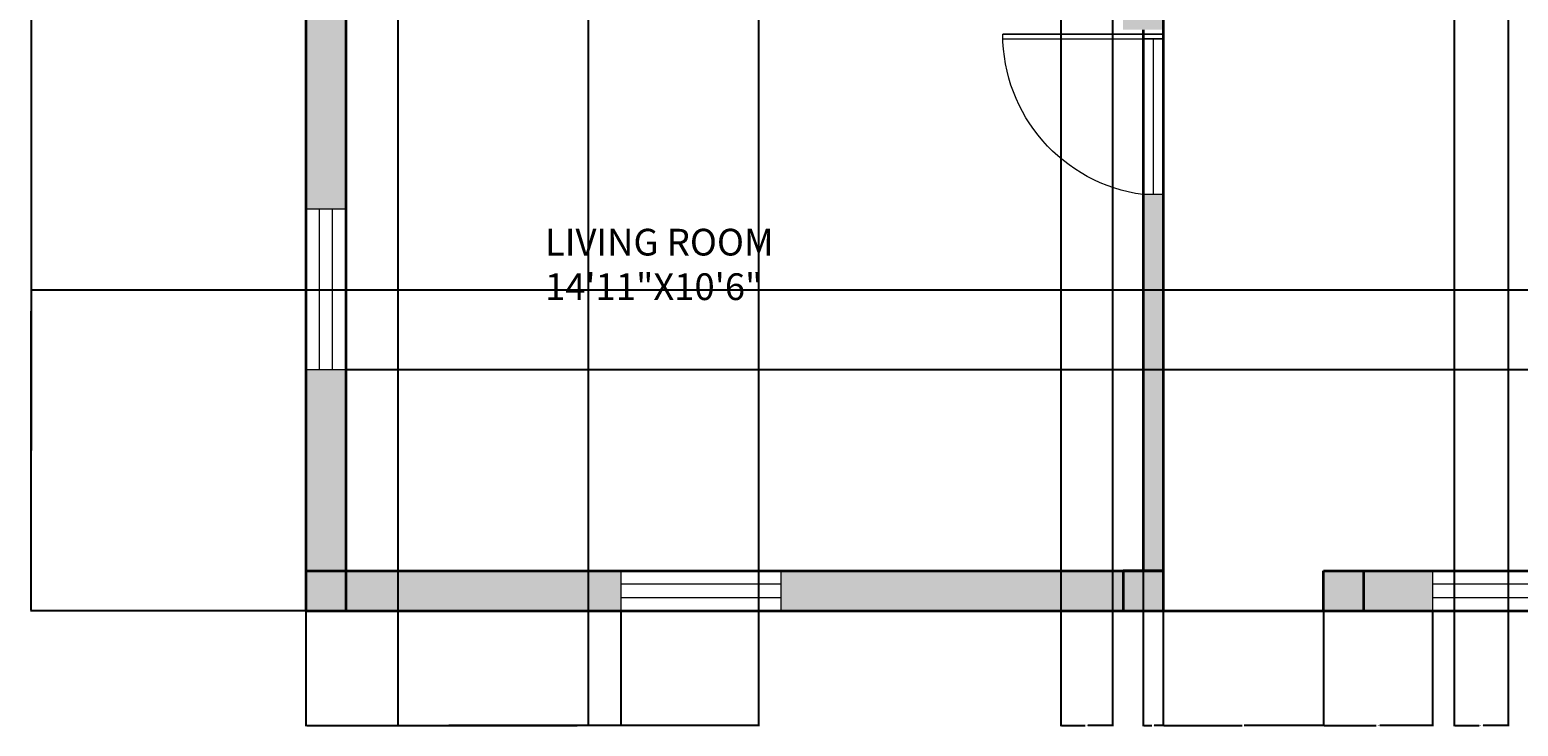
# Model space of a CAD drawing. Units: inches. Extents: x 6217 to 6782, y 16564 to 16973.
# Tile 1 of 3: x 6218 to 6552, y 16564 to 16720. Entities that reach past the tile are written whole.
import ezdxf

# ---------------------------------------------------------------- set-up
doc = ezdxf.new("R2010")
doc.units = ezdxf.units.IN
doc.header["$MEASUREMENT"] = 0
for name, color, linetype, lineweight in [('A-ANNO-DIMS', 2, 'Continuous', 18), ('A-AREA-IDEN', 7, 'Continuous', 18), ('A-COLS', 7, 'Continuous', 35), ('A-DOOR', 3, 'Continuous', 18), ('A-GLAZ', 4, 'Continuous', 18), ('A-WALL', 7, 'Continuous', 35)]:
    doc.layers.add(name, color=color, linetype=linetype, lineweight=lineweight)
doc.layers.add('A-COLS-PATT', color=252, linetype='Continuous', lineweight=13, true_color=0x939598)
doc.layers.add('A-WALL-PATT', color=146, linetype='Continuous', lineweight=13, true_color=0x105689)
doc.styles.get("Standard").update_dxf_attribs({"font": 'arial.ttf'})
doc.dimstyles.get("Standard").update_dxf_attribs({"dimtxt": 0.18, "dimasz": 0.18, "dimexe": 0.18, "dimexo": 0.0625, "dimgap": 0.09, "dimtad": 0, "dimtih": 1, "dimtoh": 1, "dimdec": 4, "dimzin": 0, "dimdsep": 46, "dimtxsty": 'Standard', "dimcen": 0.09, "dimadec": 0, "dimazin": 0, "dimtfac": 1, "dimtdec": 4, "dimtofl": 0, "dimtmove": 0, "dimatfit": 3, "dimfxl": 1, "dimtolj": 1, "dimtzin": 0, "dimarcsym": 0})

# ---------------------------------------------------------------- blocks, each defined once
blk = doc.blocks.new('WIN-36')
for p, q in [((0, 9), (0, 0)), ((36, 9), (0, 9)), ((36, 0), (36, 9)), ((36, 6), (0, 6)), ((0, 3), (36, 3)), ((0, 0), (36, 0))]:
    blk.add_line(p, q)
blk = doc.blocks.new('DOOR-SINGLE-36-A')
for p, q in [((0, 36), (-4.5, 36)), ((-2.25, 1), (-2.25, 36)), ((0, 0), (0, 36)), ((-36, 1), (0, 1)), ((0, 0), (-36, 0)), ((-36, 0), (0, 0)), ((0, 1), (-4.5, 1)), ((-4.5, 1), (-2.25, 1)), ((0, -1), (0, 0))]:
    blk.add_line(p, q)
blk.add_arc((0.32, 0), 36.32, 97.6281, 180)
blk = doc.blocks.new('*D20')
at = {"layer": 'A-ANNO-DIMS', "color": 0, "lineweight": -2, "transparency": 16777216}
for p, q in [((6279.47, 16724.5), (6217.65, 16724.5)), ((6217.83, 16724.32), (6217.83, 16657.19)), ((6217.83, 16589.68), (6217.83, 16656.82)), ((6279.47, 16589.5), (6217.65, 16589.5))]:
    blk.add_line(p, q, dxfattribs=at)
at = {"layer": 'A-ANNO-DIMS', "color": 0, "transparency": 16777216}
for points in [[(6217.8, 16724.32), (6217.86, 16724.32), (6217.83, 16724.5)], [(6217.8, 16589.68), (6217.86, 16589.68), (6217.83, 16589.5)]]:
    blk.add_solid(points, dxfattribs=at)
at = {"layer": 'Defpoints', "color": 0, "transparency": 16777216}
for p in [(6217.83, 16724.5), (6279.53, 16724.5), (6279.53, 16589.5)]:
    blk.add_point(p, dxfattribs=at)
at = {"layer": 'A-ANNO-DIMS', "color": 0, "transparency": 16777216, "insert": (6217.83, 16657), "char_height": 0.18, "attachment_point": 5}
blk.add_mtext('\\A1;135', dxfattribs=at)
blk = doc.blocks.new('*D21')
at = {"layer": 'A-ANNO-DIMS', "color": 0, "lineweight": -2, "transparency": 16777216}
for p, q in [((6279.53, 16937.94), (6279.53, 16563.62)), ((6342.94, 16937.94), (6342.94, 16563.62)), ((6279.71, 16563.8), (6310.86, 16563.8)), ((6342.76, 16563.8), (6311.61, 16563.8))]:
    blk.add_line(p, q, dxfattribs=at)
at = {"layer": 'A-ANNO-DIMS', "color": 0, "transparency": 16777216}
for points in [[(6279.71, 16563.83), (6279.71, 16563.77), (6279.53, 16563.8)], [(6342.76, 16563.83), (6342.76, 16563.77), (6342.94, 16563.8)]]:
    blk.add_solid(points, dxfattribs=at)
at = {"layer": 'Defpoints', "color": 0, "transparency": 16777216}
for p in [(6279.53, 16938), (6342.94, 16938), (6342.94, 16563.8)]:
    blk.add_point(p, dxfattribs=at)
at = {"layer": 'A-ANNO-DIMS', "color": 0, "transparency": 16777216, "insert": (6311.23, 16563.8), "char_height": 0.18, "attachment_point": 5}
blk.add_mtext('\\A1;63.41', dxfattribs=at)
blk = doc.blocks.new('*D22')
at = {"layer": 'A-ANNO-DIMS', "color": 0, "lineweight": -2, "transparency": 16777216}
for p, q in [((6449.03, 16937.94), (6449.03, 16563.62)), ((6460.63, 16937.94), (6460.63, 16563.62)), ((6449.21, 16563.8), (6454.51, 16563.8)), ((6460.45, 16563.8), (6455.14, 16563.8))]:
    blk.add_line(p, q, dxfattribs=at)
at = {"layer": 'A-ANNO-DIMS', "color": 0, "transparency": 16777216}
for points in [[(6449.21, 16563.83), (6449.21, 16563.77), (6449.03, 16563.8)], [(6460.45, 16563.83), (6460.45, 16563.77), (6460.63, 16563.8)]]:
    blk.add_solid(points, dxfattribs=at)
at = {"layer": 'Defpoints', "color": 0, "transparency": 16777216}
for p in [(6449.03, 16938), (6460.63, 16938), (6460.63, 16563.8)]:
    blk.add_point(p, dxfattribs=at)
at = {"layer": 'A-ANNO-DIMS', "color": 0, "transparency": 16777216, "insert": (6454.83, 16563.8), "char_height": 0.18, "attachment_point": 5}
blk.add_mtext('\\A1;11.6', dxfattribs=at)
blk = doc.blocks.new('*D23')
at = {"layer": 'A-ANNO-DIMS', "color": 0, "lineweight": -2, "transparency": 16777216}
for p, q in [((6537.38, 16937.94), (6537.38, 16563.62)), ((6549.53, 16937.94), (6549.53, 16563.62)), ((6537.56, 16563.8), (6543, 16563.8)), ((6549.35, 16563.8), (6543.91, 16563.8))]:
    blk.add_line(p, q, dxfattribs=at)
at = {"layer": 'A-ANNO-DIMS', "color": 0, "transparency": 16777216}
for points in [[(6537.56, 16563.83), (6537.56, 16563.77), (6537.38, 16563.8)], [(6549.35, 16563.83), (6549.35, 16563.77), (6549.53, 16563.8)]]:
    blk.add_solid(points, dxfattribs=at)
at = {"layer": 'Defpoints', "color": 0, "transparency": 16777216}
for p in [(6537.38, 16938), (6549.53, 16938), (6549.53, 16563.8)]:
    blk.add_point(p, dxfattribs=at)
at = {"layer": 'A-ANNO-DIMS', "color": 0, "transparency": 16777216, "insert": (6543.45, 16563.8), "char_height": 0.18, "attachment_point": 5}
blk.add_mtext('\\A1;12.147', dxfattribs=at)
blk = doc.blocks.new('*D27')
at = {"layer": 'A-ANNO-DIMS', "color": 0, "lineweight": -2, "transparency": 16777216}
for p, q in [((6746.47, 16661.53), (6217.65, 16661.53)), ((6217.83, 16661.35), (6217.83, 16625.7)), ((6217.83, 16589.68), (6217.83, 16625.33)), ((6746.47, 16589.5), (6217.65, 16589.5))]:
    blk.add_line(p, q, dxfattribs=at)
at = {"layer": 'A-ANNO-DIMS', "color": 0, "transparency": 16777216}
for points in [[(6217.8, 16661.35), (6217.86, 16661.35), (6217.83, 16661.53)], [(6217.8, 16589.68), (6217.86, 16589.68), (6217.83, 16589.5)]]:
    blk.add_solid(points, dxfattribs=at)
at = {"layer": 'Defpoints', "color": 0, "transparency": 16777216}
for p in [(6217.83, 16661.53), (6746.53, 16661.53), (6746.53, 16589.5)]:
    blk.add_point(p, dxfattribs=at)
at = {"layer": 'A-ANNO-DIMS', "color": 0, "transparency": 16777216, "insert": (6217.83, 16625.52), "char_height": 0.18, "attachment_point": 5}
blk.add_mtext('\\A1;72.03', dxfattribs=at)
blk = doc.blocks.new('*D28')
at = {"layer": 'A-ANNO-DIMS', "color": 0, "lineweight": -2, "transparency": 16777216}
for p, q in [((6288.59, 16643.72), (6781.41, 16643.72)), ((6781.23, 16643.54), (6781.23, 16616.79)), ((6781.23, 16589.68), (6781.23, 16616.43)), ((6288.59, 16589.5), (6781.41, 16589.5))]:
    blk.add_line(p, q, dxfattribs=at)
at = {"layer": 'A-ANNO-DIMS', "color": 0, "transparency": 16777216}
for points in [[(6781.2, 16643.54), (6781.26, 16643.54), (6781.23, 16643.72)], [(6781.2, 16589.68), (6781.26, 16589.68), (6781.23, 16589.5)]]:
    blk.add_solid(points, dxfattribs=at)
at = {"layer": 'Defpoints', "color": 0, "transparency": 16777216}
for p in [(6288.53, 16643.72), (6781.23, 16643.72), (6288.53, 16589.5)]:
    blk.add_point(p, dxfattribs=at)
at = {"layer": 'A-ANNO-DIMS', "color": 0, "transparency": 16777216, "insert": (6781.23, 16616.61), "char_height": 0.18, "attachment_point": 5}
blk.add_mtext('\\A1;54.22', dxfattribs=at)
blk = doc.blocks.new('*D29')
at = {"layer": 'A-ANNO-DIMS', "color": 0, "lineweight": -2, "transparency": 16777216}
for p, q in [((6279.53, 16589.44), (6279.53, 16563.62)), ((6350.27, 16589.44), (6350.27, 16563.62)), ((6279.71, 16563.8), (6314.51, 16563.8)), ((6350.09, 16563.8), (6315.29, 16563.8))]:
    blk.add_line(p, q, dxfattribs=at)
at = {"layer": 'A-ANNO-DIMS', "color": 0, "transparency": 16777216}
for points in [[(6279.71, 16563.83), (6279.71, 16563.77), (6279.53, 16563.8)], [(6350.09, 16563.83), (6350.09, 16563.77), (6350.27, 16563.8)]]:
    blk.add_solid(points, dxfattribs=at)
at = {"layer": 'Defpoints', "color": 0, "transparency": 16777216}
for p in [(6279.53, 16589.5), (6350.27, 16589.5), (6350.27, 16563.8)]:
    blk.add_point(p, dxfattribs=at)
at = {"layer": 'A-ANNO-DIMS', "color": 0, "transparency": 16777216, "insert": (6314.9, 16563.8), "char_height": 0.18, "attachment_point": 5}
blk.add_mtext('\\A1;70.74', dxfattribs=at)
blk = doc.blocks.new('*D30')
at = {"layer": 'A-ANNO-DIMS', "color": 0, "lineweight": -2, "transparency": 16777216}
for p, q in [((6472.03, 16589.44), (6472.03, 16563.62)), ((6508.03, 16589.44), (6508.03, 16563.62)), ((6472.21, 16563.8), (6489.81, 16563.8)), ((6507.85, 16563.8), (6490.25, 16563.8))]:
    blk.add_line(p, q, dxfattribs=at)
at = {"layer": 'A-ANNO-DIMS', "color": 0, "transparency": 16777216}
for points in [[(6472.21, 16563.83), (6472.21, 16563.77), (6472.03, 16563.8)], [(6507.85, 16563.83), (6507.85, 16563.77), (6508.03, 16563.8)]]:
    blk.add_solid(points, dxfattribs=at)
at = {"layer": 'Defpoints', "color": 0, "transparency": 16777216}
for p in [(6472.03, 16589.5), (6508.03, 16589.5), (6508.03, 16563.8)]:
    blk.add_point(p, dxfattribs=at)
at = {"layer": 'A-ANNO-DIMS', "color": 0, "transparency": 16777216, "insert": (6490.03, 16563.8), "char_height": 0.18, "attachment_point": 5}
blk.add_mtext('\\A1;36', dxfattribs=at)
blk = doc.blocks.new('*D31')
at = {"layer": 'A-ANNO-DIMS', "color": 0, "lineweight": -2, "transparency": 16777216}
for p, q in [((6508.03, 16589.44), (6508.03, 16563.62)), ((6532.52, 16589.44), (6532.52, 16563.62)), ((6508.21, 16563.8), (6519.88, 16563.8)), ((6532.34, 16563.8), (6520.67, 16563.8))]:
    blk.add_line(p, q, dxfattribs=at)
at = {"layer": 'A-ANNO-DIMS', "color": 0, "transparency": 16777216}
for points in [[(6508.21, 16563.83), (6508.21, 16563.77), (6508.03, 16563.8)], [(6532.34, 16563.83), (6532.34, 16563.77), (6532.52, 16563.8)]]:
    blk.add_solid(points, dxfattribs=at)
at = {"layer": 'Defpoints', "color": 0, "transparency": 16777216}
for p in [(6508.03, 16589.5), (6532.52, 16589.5), (6532.52, 16563.8)]:
    blk.add_point(p, dxfattribs=at)
at = {"layer": 'A-ANNO-DIMS', "color": 0, "transparency": 16777216, "insert": (6520.27, 16563.8), "char_height": 0.18, "attachment_point": 5}
blk.add_mtext('\\A1;24.49', dxfattribs=at)
blk = doc.blocks.new('*D37')
at = {"layer": 'A-ANNO-DIMS', "color": 0, "lineweight": -2, "transparency": 16777216}
for p, q in [((6300.17, 16774.19), (6300.17, 16563.62)), ((6381.17, 16774.19), (6381.17, 16563.62)), ((6300.35, 16563.8), (6340.47, 16563.8)), ((6380.99, 16563.8), (6340.88, 16563.8))]:
    blk.add_line(p, q, dxfattribs=at)
at = {"layer": 'A-ANNO-DIMS', "color": 0, "transparency": 16777216}
for points in [[(6300.35, 16563.83), (6300.35, 16563.77), (6300.17, 16563.8)], [(6380.99, 16563.83), (6380.99, 16563.77), (6381.17, 16563.8)]]:
    blk.add_solid(points, dxfattribs=at)
at = {"layer": 'Defpoints', "color": 0, "transparency": 16777216}
for p in [(6300.17, 16774.25), (6381.17, 16774.25), (6381.17, 16563.8)]:
    blk.add_point(p, dxfattribs=at)
at = {"layer": 'A-ANNO-DIMS', "color": 0, "transparency": 16777216, "insert": (6340.67, 16563.8), "char_height": 0.18, "attachment_point": 5}
blk.add_mtext('\\A1;81', dxfattribs=at)
blk = doc.blocks.new('*D40')
at = {"layer": 'A-ANNO-DIMS', "color": 0, "lineweight": -2, "transparency": 16777216}
for p, q in [((6467.53, 16682.94), (6467.53, 16563.62)), ((6472.03, 16682.94), (6472.03, 16563.62)), ((6467.71, 16563.8), (6469.52, 16563.8)), ((6471.85, 16563.8), (6470.04, 16563.8))]:
    blk.add_line(p, q, dxfattribs=at)
at = {"layer": 'A-ANNO-DIMS', "color": 0, "transparency": 16777216}
for points in [[(6467.71, 16563.83), (6467.71, 16563.77), (6467.53, 16563.8)], [(6471.85, 16563.83), (6471.85, 16563.77), (6472.03, 16563.8)]]:
    blk.add_solid(points, dxfattribs=at)
at = {"layer": 'Defpoints', "color": 0, "transparency": 16777216}
for p in [(6467.53, 16683), (6472.03, 16683), (6472.03, 16563.8)]:
    blk.add_point(p, dxfattribs=at)
at = {"layer": 'A-ANNO-DIMS', "color": 0, "transparency": 16777216, "insert": (6469.78, 16563.8), "char_height": 0.18, "attachment_point": 5}
blk.add_mtext('\\A1;4.5', dxfattribs=at)

msp = doc.modelspace()

# ---------------------------------------------------------------- hatches: boundary and pattern name
at = {"layer": 'A-COLS-PATT'}
h = msp.add_hatch(color=256, dxfattribs=at)
h.dxf.hatch_style = 1
h.paths.add_polyline_path([(6288.5285, 16947.0033), (6279.5285, 16947.0033), (6279.5285, 16938.0033), (6288.5285, 16938.0033)])
h.paths.add_polyline_path([(6449.0285, 16947.0033), (6440.0285, 16947.0033), (6440.0285, 16938.0033), (6449.0285, 16938.0033)])
h.paths.add_polyline_path([(6506.0285, 16947.0033), (6497.0285, 16947.0033), (6497.0285, 16938.0033), (6506.0285, 16938.0033)])
h.paths.add_polyline_path([(6643.0285, 16947.0033), (6634.0285, 16947.0033), (6634.0285, 16938.0033), (6643.0285, 16938.0033)])
h.paths.add_polyline_path([(6755.5285, 16947.0033), (6746.5285, 16947.0033), (6746.5285, 16938.0033), (6755.5285, 16938.0033)])
h.paths.add_polyline_path([(6755.5285, 16770.0033), (6746.5285, 16770.0033), (6746.5285, 16761.0033), (6755.5285, 16761.0033)])
h.paths.add_polyline_path([(6643.0285, 16770.0033), (6634.0285, 16770.0033), (6634.0285, 16761.0033), (6643.0285, 16761.0033)])
h.paths.add_polyline_path([(6755.5285, 16598.5033), (6746.5285, 16598.5033), (6746.5285, 16589.5033), (6755.5285, 16589.5033)])
h.paths.add_polyline_path([(6643.0285, 16598.5033), (6634.0285, 16598.5033), (6634.0285, 16589.5033), (6643.0285, 16589.5033)])
h.paths.add_polyline_path([(6517.0285, 16598.5033), (6508.0285, 16598.5033), (6508.0285, 16589.5033), (6517.0285, 16589.5033)])
h.paths.add_polyline_path([(6472.0285, 16598.5033), (6463.0285, 16598.5033), (6463.0285, 16589.5033), (6472.0285, 16589.5033)])
h.paths.add_polyline_path([(6472.0285, 16729.0033), (6463.0285, 16729.0033), (6463.0285, 16720.0033), (6472.0285, 16720.0033)])
h.paths.add_polyline_path([(6288.5285, 16598.5033), (6279.5285, 16598.5033), (6279.5285, 16589.5033), (6288.5285, 16589.5033)])
h.paths.add_polyline_path([(6288.5285, 16729.0033), (6279.5285, 16729.0033), (6279.5285, 16720.0033), (6288.5285, 16720.0033)])
h.paths.add_polyline_path([(6288.5285, 16812.0033), (6279.5285, 16812.0033), (6279.5285, 16803.0033), (6288.5285, 16803.0033)])
h.paths.add_polyline_path([(6449.0285, 16812.0033), (6440.0285, 16812.0033), (6440.0285, 16803.0033), (6449.0285, 16803.0033)])
at = {"layer": 'A-WALL-PATT'}
h = msp.add_hatch(color=256, dxfattribs=at)
h.dxf.hatch_style = 1
h.paths.add_polyline_path([(6497.0285, 16947.0033), (6484.6293, 16947.0033), (6484.6293, 16938.0033), (6497.0285, 16938.0033)])
h.paths.add_polyline_path([(6513.3814, 16947.0033), (6506.0285, 16947.0033), (6506.0285, 16938.0033), (6513.3814, 16938.0033)])
h.paths.add_polyline_path([(6572.828, 16947.0033), (6537.3814, 16947.0033), (6537.3814, 16938.0033), (6549.5285, 16938.0033), (6549.5285, 16812.0033), (6534.5285, 16812.0033), (6534.5285, 16807.5033), (6597.0285, 16807.5033), (6597.0285, 16812.0033), (6554.0285, 16812.0033), (6554.0285, 16938.0033), (6572.828, 16938.0033)])
h.paths.add_polyline_path([(6501.5285, 16938.0033), (6497.0285, 16938.0033), (6497.0285, 16854.0033), (6449.0285, 16854.0033), (6449.0285, 16855.0033), (6444.5285, 16855.0033), (6444.5285, 16854.0033), (6444.5285, 16849.0033), (6449.0285, 16849.0033), (6449.0285, 16849.5033), (6497.0285, 16849.5033), (6497.0285, 16807.5033), (6502.5285, 16807.5033), (6502.5285, 16812.0033), (6501.5285, 16812.0033)])
h.paths.add_polyline_path([(6634.0285, 16947.0033), (6608.828, 16947.0033), (6608.828, 16938.0033), (6634.0285, 16938.0033)])
h.paths.add_polyline_path([(6664.4385, 16947.0033), (6643.0285, 16947.0033), (6643.0285, 16938.0033), (6664.4385, 16938.0033)])
h.paths.add_polyline_path([(6638.5285, 16938.0033), (6634.0285, 16938.0033), (6634.0285, 16812.0033), (6633.0285, 16812.0033), (6633.0285, 16807.5033), (6634.0285, 16807.5033), (6634.0285, 16807.0033), (6638.5285, 16807.0033)])
h.paths.add_polyline_path([(6746.5285, 16947.0033), (6700.4385, 16947.0033), (6700.4385, 16938.0033), (6746.5285, 16938.0033)])
h.paths.add_polyline_path([(6755.5285, 16938.0033), (6746.5285, 16938.0033), (6746.5285, 16895.525), (6755.5285, 16895.525)])
h.paths.add_polyline_path([(6755.5285, 16859.525), (6746.5285, 16859.525), (6746.5285, 16770.0033), (6755.5285, 16770.0033)])
h.paths.add_polyline_path([(6746.5285, 16770.0033), (6643.0285, 16770.0033), (6643.0285, 16765.5033), (6746.5285, 16765.5033)])
h.paths.add_polyline_path([(6755.5285, 16761.0033), (6746.5285, 16761.0033), (6746.5285, 16697.5292), (6755.5285, 16697.5292)])
h.paths.add_polyline_path([(6440.0285, 16812.0033), (6288.5285, 16812.0033), (6288.5285, 16807.5033), (6440.0285, 16807.5033)])
h.paths.add_polyline_path([(6288.5285, 16938.0033), (6279.5285, 16938.0033), (6279.5285, 16849.0033), (6288.5285, 16849.0033)])
h.paths.add_polyline_path([(6279.5285, 16729.0033), (6248.0285, 16729.0033), (6248.0285, 16807.5033), (6279.5285, 16807.5033), (6279.5285, 16812.0033), (6243.5285, 16812.0033), (6243.5285, 16724.5033), (6279.5285, 16724.5033)])
h.paths.add_polyline_path([(6463.0285, 16729.0033), (6288.5285, 16729.0033), (6288.5285, 16724.5033), (6463.0285, 16724.5033)])
h.paths.add_polyline_path([(6288.5285, 16720.0033), (6279.5285, 16720.0033), (6279.5285, 16679.7207), (6288.5285, 16679.7207)])
h.paths.add_polyline_path([(6288.5285, 16643.7207), (6279.5285, 16643.7207), (6279.5285, 16598.5033), (6288.5285, 16598.5033)])
h.paths.add_polyline_path([(6350.2697, 16598.5033), (6288.5285, 16598.5033), (6288.5285, 16589.5033), (6350.2697, 16589.5033)])
h.paths.add_polyline_path([(6463.0285, 16598.5033), (6386.2697, 16598.5033), (6386.2697, 16589.5033), (6463.0285, 16589.5033)])
h.paths.add_polyline_path([(6472.0285, 16683.0033), (6467.5285, 16683.0033), (6467.5285, 16598.5033), (6472.0285, 16598.5033)])
h.paths.add_polyline_path([(6532.5191, 16598.5033), (6517.0285, 16598.5033), (6517.0285, 16589.5033), (6532.5191, 16589.5033)])
h.paths.add_polyline_path([(6634.0285, 16598.5033), (6568.5191, 16598.5033), (6568.5191, 16589.5033), (6634.0285, 16589.5033)])
h.paths.add_polyline_path([(6661.0648, 16598.5033), (6643.0285, 16598.5033), (6643.0285, 16589.5033), (6661.0648, 16589.5033)])
h.paths.add_polyline_path([(6746.5285, 16598.5033), (6697.0648, 16598.5033), (6697.0648, 16589.5033), (6746.5285, 16589.5033)])
h.paths.add_polyline_path([(6755.5285, 16661.5292), (6746.5285, 16661.5292), (6746.5285, 16598.5033), (6755.5285, 16598.5033)])
h.paths.add_polyline_path([(6638.5285, 16724.0033), (6634.0285, 16724.0033), (6634.0285, 16598.5033), (6638.5285, 16598.5033)])

# ---------------------------------------------------------------- linework, layer by layer
at = {"layer": 'A-COLS'}
for p, q in [((6472.0285, 16598.5033), (6463.0285, 16598.5033)), ((6463.0285, 16598.5033), (6463.0285, 16589.5033)), ((6508.0285, 16589.5033), (6508.0285, 16598.5033)), ((6508.0285, 16598.5033), (6517.0285, 16598.5033)), ((6517.0285, 16598.5033), (6517.0285, 16589.5033)), ((6463.0285, 16589.5033), (6472.0285, 16589.5033))]:
    msp.add_line(p, q, dxfattribs=at)
at = {"layer": 'A-WALL'}
for p, q in [((6279.5285, 16729.0033), (6279.5285, 16589.5033)), ((6288.5285, 16729.0033), (6288.5285, 16589.5033)), ((6472.0285, 16729.0033), (6472.0285, 16589.5033)), ((6467.5285, 16720.0033), (6467.5285, 16598.5033)), ((6279.5285, 16598.5033), (6472.0285, 16598.5033)), ((6508.0285, 16598.5033), (6755.5285, 16598.5033)), ((6279.5285, 16589.5033), (6755.5285, 16589.5033)), ((6472.0285, 16589.5033), (6508.0285, 16589.5033))]:
    msp.add_line(p, q, dxfattribs=at)

# ---------------------------------------------------------------- block references
at = {"layer": 'A-DOOR', "extrusion": (0, 0, -1), "zscale": -1, "rotation": 180}
msp.add_blockref('DOOR-SINGLE-36-A', (-6472.0285, 16719.0033), dxfattribs=at)
at = {"layer": 'A-GLAZ', "rotation": 270.0000000000055}
msp.add_blockref('WIN-36', (6279.5285, 16679.7207), dxfattribs=at)
at = {"layer": 'A-GLAZ'}
for p in [(6350.2697, 16589.5033), (6532.5191, 16589.5033)]:
    msp.add_blockref('WIN-36', p, dxfattribs=at)

# ---------------------------------------------------------------- texts
at = {"layer": 'A-AREA-IDEN', "insert": (6333.2268, 16675.3159), "char_height": 6, "attachment_point": 1}
msp.add_mtext_dynamic_manual_height_columns('LIVING ROOM \\P14\'11"X10\'6"', width=71.707741, gutter_width=1, heights=[0], dxfattribs=at)

# ---------------------------------------------------------------- dimensions: what is measured, and where the dimension line sits
at = {"layer": 'A-ANNO-DIMS'}
for base, p1, p2, override, picture, middle in [((6342.9367, 16563.8008), (6279.5285, 16938.0033), (6342.9367, 16938.0033), {"dimdec": 2, "dimlfac": 1, "dimrnd": 0, "dimzin": 0, "dimdsep": 46, "dimlunit": 2}, '*D21', (6311.2326, 16563.8008)), ((6460.6293, 16563.8008), (6449.0285, 16938.0033), (6460.6293, 16938.0033), {"dimdec": 1, "dimlfac": 1, "dimrnd": 0, "dimzin": 0, "dimdsep": 46, "dimlunit": 2}, '*D22', (6454.8289, 16563.8008)), ((6549.5285, 16563.8008), (6537.3814, 16938.0033), (6549.5285, 16938.0033), {"dimdec": 3, "dimlfac": 1, "dimrnd": 0, "dimzin": 0, "dimdsep": 46, "dimlunit": 2}, '*D23', (6543.4549, 16563.8008)), ((6381.174, 16563.8008), (6300.174, 16774.2533), (6381.174, 16774.2533), {"dimdec": 0, "dimlfac": 1, "dimrnd": 0, "dimzin": 0, "dimdsep": 46, "dimlunit": 2}, '*D37', (6340.674, 16563.8008)), ((6472.0285, 16563.8008), (6467.5285, 16683.0033), (6472.0285, 16683.0033), {"dimdec": 1, "dimlfac": 1, "dimrnd": 0, "dimzin": 0, "dimdsep": 46, "dimlunit": 2}, '*D40', (6469.7785, 16563.8008)), ((6350.2697, 16563.8008), (6279.5285, 16589.5033), (6350.2697, 16589.5033), {"dimdec": 2, "dimlfac": 1, "dimrnd": 0, "dimzin": 0, "dimdsep": 46, "dimlunit": 2}, '*D29', (6314.8991, 16563.8008)), ((6508.0285, 16563.8008), (6472.0285, 16589.5033), (6508.0285, 16589.5033), {"dimdec": 0, "dimlfac": 1, "dimrnd": 0, "dimzin": 0, "dimdsep": 46, "dimlunit": 2}, '*D30', (6490.0285, 16563.8008)), ((6532.5191, 16563.8008), (6508.0285, 16589.5033), (6532.5191, 16589.5033), {"dimdec": 2, "dimlfac": 1, "dimrnd": 0, "dimzin": 0, "dimdsep": 46, "dimlunit": 2}, '*D31', (6520.2738, 16563.8008))]:
    dim = msp.add_linear_dim(base=base, p1=p1, p2=p2, dimstyle='Standard', override=override, dxfattribs=at)
    dim.commit()
    dim.dimension.update_dxf_attribs({"geometry": picture, "text_midpoint": middle})
for base, p1, p2, override, picture, middle in [((6217.826, 16724.5033), (6279.5285, 16589.5033), (6279.5285, 16724.5033), {"dimdec": 0, "dimlfac": 1, "dimrnd": 0, "dimzin": 0, "dimdsep": 46, "dimlunit": 2}, '*D20', (6217.826, 16657.0033)), ((6217.826, 16661.5292), (6746.5285, 16589.5033), (6746.5285, 16661.5292), {"dimdec": 2, "dimlfac": 1, "dimrnd": 0, "dimzin": 0, "dimdsep": 46, "dimlunit": 2}, '*D27', (6217.826, 16625.5162)), ((6781.231, 16643.7207), (6288.5285, 16589.5033), (6288.5285, 16643.7207), {"dimdec": 2, "dimlfac": 1, "dimrnd": 0, "dimzin": 0, "dimdsep": 46, "dimlunit": 2}, '*D28', (6781.231, 16616.612))]:
    dim = msp.add_linear_dim(base=base, p1=p1, p2=p2, angle=90, dimstyle='Standard', override=override, dxfattribs=at)
    dim.commit()
    dim.dimension.update_dxf_attribs({"geometry": picture, "text_midpoint": middle})

doc.saveas('drawing.dxf')
